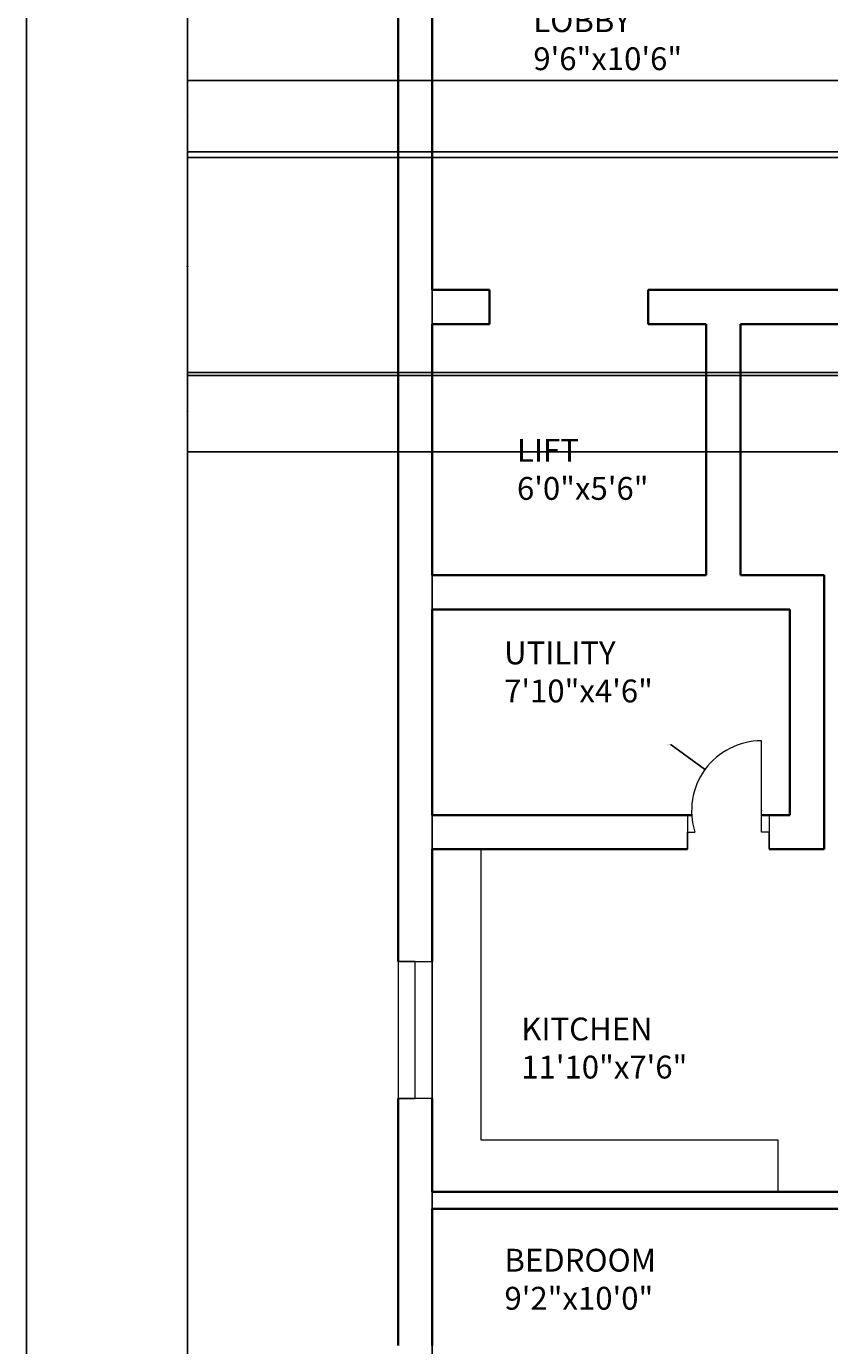
# Model space of a CAD drawing. Units: inches. Extents: x 1902 to 2626, y 1199 to 2408.
# Tile 2 of 9: x 1902 to 2113, y 1470 to 1817. Entities that reach past the tile are written whole.
import ezdxf

# ---------------------------------------------------------------- set-up
doc = ezdxf.new("R2010")
doc.units = ezdxf.units.IN
for name, color, linetype, lineweight in [('A-ANNO-DIMS', 2, 'Continuous', 18), ('A-ANNO-TTLB', 7, 'Continuous', 25), ('A-AREA-IDEN', 7, 'Continuous', 18), ('A-DOOR', 31, 'Continuous', 18), ('A-FLOR-CASE', 8, 'Continuous', 18), ('A-GLAZ', 181, 'Continuous', 18), ('A-WALL', 7, 'Continuous', 35)]:
    doc.layers.add(name, color=color, linetype=linetype, lineweight=lineweight)
doc.styles.get("Standard").update_dxf_attribs({"font": 'arial.ttf'})
doc.dimstyles.get("Standard").update_dxf_attribs({"dimtxt": 0.18, "dimasz": 0.18, "dimexe": 0.18, "dimexo": 0.0625, "dimgap": 0.09, "dimtad": 0, "dimtih": 1, "dimtoh": 1, "dimdec": 4, "dimzin": 0, "dimdsep": 46, "dimtxsty": 'Standard', "dimcen": 0.09, "dimadec": 0, "dimazin": 0, "dimtfac": 1, "dimtdec": 4, "dimtofl": 0, "dimtmove": 0, "dimatfit": 3, "dimfxl": 1, "dimtolj": 1, "dimtzin": 0, "dimarcsym": 0})

# ---------------------------------------------------------------- blocks, each defined once
blk = doc.blocks.new('*D29')
at = {"layer": 'A-ANNO-DIMS', "color": 0, "lineweight": -2, "transparency": 16777216}
for p, q in [((2191.29, 2322.47), (1943.87, 2322.47)), ((1944.05, 2322.29), (1944.05, 1836.38)), ((1944.05, 1350.11), (1944.05, 1836.02)), ((2202.79, 1349.93), (1943.87, 1349.93))]:
    blk.add_line(p, q, dxfattribs=at)
at = {"layer": 'A-ANNO-DIMS', "color": 0, "transparency": 16777216}
for points in [[(1944.02, 2322.29), (1944.08, 2322.29), (1944.05, 2322.47)], [(1944.02, 1350.11), (1944.08, 1350.11), (1944.05, 1349.93)]]:
    blk.add_solid(points, dxfattribs=at)
at = {"layer": 'Defpoints', "color": 0, "transparency": 16777216}
for p in [(1944.05, 2322.47), (2191.35, 2322.47), (2202.85, 1349.93)]:
    blk.add_point(p, dxfattribs=at)
at = {"layer": 'A-ANNO-DIMS', "color": 0, "transparency": 16777216, "insert": (1944.05, 1836.2), "char_height": 0.18, "attachment_point": 5}
blk.add_mtext('\\A1;972.5', dxfattribs=at)
blk = doc.blocks.new('*D38')
at = {"layer": 'A-ANNO-DIMS', "color": 0, "lineweight": -2, "transparency": 16777216}
for p, q in [((2008.35, 1874.05), (2008.35, 1198.67)), ((2128.35, 1874.05), (2128.35, 1198.67)), ((2008.53, 1198.85), (2068.07, 1198.85)), ((2128.17, 1198.85), (2068.63, 1198.85))]:
    blk.add_line(p, q, dxfattribs=at)
at = {"layer": 'A-ANNO-DIMS', "color": 0, "transparency": 16777216}
for points in [[(2008.53, 1198.88), (2008.53, 1198.82), (2008.35, 1198.85)], [(2128.17, 1198.88), (2128.17, 1198.82), (2128.35, 1198.85)]]:
    blk.add_solid(points, dxfattribs=at)
at = {"layer": 'Defpoints', "color": 0, "transparency": 16777216}
for p in [(2008.35, 1874.11), (2128.35, 1874.11), (2128.35, 1198.85)]:
    blk.add_point(p, dxfattribs=at)
at = {"layer": 'A-ANNO-DIMS', "color": 0, "transparency": 16777216, "insert": (2068.35, 1198.85), "char_height": 0.18, "attachment_point": 5}
blk.add_mtext('\\A1;120', dxfattribs=at)
blk = doc.blocks.new('*D40')
at = {"layer": 'A-ANNO-DIMS', "color": 0, "lineweight": -2, "transparency": 16777216}
for p, q in [((2313.55, 1782.51), (1943.87, 1782.51)), ((1944.05, 1782.33), (1944.05, 1754.03)), ((1944.05, 1725.38), (1944.05, 1753.67)), ((2313.55, 1725.2), (1943.87, 1725.2))]:
    blk.add_line(p, q, dxfattribs=at)
at = {"layer": 'A-ANNO-DIMS', "color": 0, "transparency": 16777216}
for points in [[(1944.02, 1782.33), (1944.08, 1782.33), (1944.05, 1782.51)], [(1944.02, 1725.38), (1944.08, 1725.38), (1944.05, 1725.2)]]:
    blk.add_solid(points, dxfattribs=at)
at = {"layer": 'Defpoints', "color": 0, "transparency": 16777216}
for p in [(1944.05, 1782.51), (2313.62, 1782.51), (2313.62, 1725.2)]:
    blk.add_point(p, dxfattribs=at)
at = {"layer": 'A-ANNO-DIMS', "color": 0, "transparency": 16777216, "insert": (1944.05, 1753.85), "char_height": 0.18, "attachment_point": 5}
blk.add_mtext('\\A1;57.31', dxfattribs=at)
blk = doc.blocks.new('*D42')
at = {"layer": 'A-ANNO-DIMS', "color": 0, "lineweight": -2, "transparency": 16777216}
for p, q in [((2267.32, 1726.02), (1943.87, 1726.02)), ((1944.05, 1725.84), (1944.05, 1715.78)), ((1944.05, 1705.36), (1944.05, 1715.41)), ((2267.32, 1705.18), (1943.87, 1705.18))]:
    blk.add_line(p, q, dxfattribs=at)
at = {"layer": 'A-ANNO-DIMS', "color": 0, "transparency": 16777216}
for points in [[(1944.02, 1725.84), (1944.08, 1725.84), (1944.05, 1726.02)], [(1944.02, 1705.36), (1944.08, 1705.36), (1944.05, 1705.18)]]:
    blk.add_solid(points, dxfattribs=at)
at = {"layer": 'Defpoints', "color": 0, "transparency": 16777216}
for p in [(1944.05, 1726.02), (2267.38, 1726.02), (2267.38, 1705.18)]:
    blk.add_point(p, dxfattribs=at)
at = {"layer": 'A-ANNO-DIMS', "color": 0, "transparency": 16777216, "insert": (1944.05, 1715.6), "char_height": 0.18, "attachment_point": 5}
blk.add_mtext('\\A1;20.84', dxfattribs=at)
blk = doc.blocks.new('*D44')
at = {"layer": 'A-ANNO-DIMS', "color": 0, "lineweight": -2, "transparency": 16777216}
for p, q in [((2265.36, 1802.76), (1943.87, 1802.76)), ((1944.05, 1802.58), (1944.05, 1793.54)), ((1944.05, 1784.15), (1944.05, 1793.18)), ((2265.36, 1783.97), (1943.87, 1783.97))]:
    blk.add_line(p, q, dxfattribs=at)
at = {"layer": 'A-ANNO-DIMS', "color": 0, "transparency": 16777216}
for points in [[(1944.02, 1802.58), (1944.08, 1802.58), (1944.05, 1802.76)], [(1944.02, 1784.15), (1944.08, 1784.15), (1944.05, 1783.97)]]:
    blk.add_solid(points, dxfattribs=at)
at = {"layer": 'Defpoints', "color": 0, "transparency": 16777216}
for p in [(1944.05, 1802.76), (2265.42, 1802.76), (2265.42, 1783.97)]:
    blk.add_point(p, dxfattribs=at)
at = {"layer": 'A-ANNO-DIMS', "color": 0, "transparency": 16777216, "insert": (1944.05, 1793.36), "char_height": 0.18, "attachment_point": 5}
blk.add_mtext('\\A1;18.79', dxfattribs=at)
blk = doc.blocks.new('*D58')
at = {"layer": 'A-ANNO-DIMS', "color": 0, "lineweight": -2, "transparency": 16777216}
for p, q in [((2070.93, 1628.13), (2071.11, 1628.13)), ((2071.11, 1628.13), (2079.87, 1621.75)), ((2094.77, 1610.85), (2094.95, 1610.85)), ((2094.86, 1610.76), (2094.86, 1610.94))]:
    blk.add_line(p, q, dxfattribs=at)
at = {"layer": 'A-ANNO-DIMS', "color": 0, "transparency": 16777216}
blk.add_solid([(2079.89, 1621.78), (2079.85, 1621.73), (2080.02, 1621.65)], dxfattribs=at)
at = {"layer": 'Defpoints', "color": 0, "transparency": 16777216}
for p in [(2080.02, 1621.65), (2094.86, 1610.85)]:
    blk.add_point(p, dxfattribs=at)
at = {"layer": 'A-ANNO-DIMS', "color": 0, "transparency": 16777216, "insert": (2070.38, 1628.13), "char_height": 0.18, "attachment_point": 5}
blk.add_mtext('\\A1;R18.356', dxfattribs=at)

msp = doc.modelspace()

# ---------------------------------------------------------------- linework, layer by layer
at = {"layer": 'A-ANNO-TTLB'}
msp.add_lwpolyline([(1901.6928, 2408.1473), (2626.1646, 2408.1473), (2626.1646, 1206.3103), (1901.6928, 1206.3103)], close=True, dxfattribs=at)
at = {"layer": 'A-DOOR'}
for p, q in [((2094.8588, 1605.2028), (2094.8588, 1629.2028)), ((2075.3921, 1609.7028), (2075.3921, 1600.7028)), ((2096.8588, 1609.7028), (2096.8588, 1600.7028)), ((2075.3921, 1600.7028), (2075.3921, 1605.2028)), ((2075.3921, 1605.2028), (2077.3921, 1605.2028)), ((2096.8588, 1605.2028), (2094.8588, 1605.2028)), ((2096.8588, 1600.7028), (2096.8588, 1605.2028))]:
    msp.add_line(p, q, dxfattribs=at)
msp.add_arc((2094.8588, 1610.8468), 18.356, 90, 197.907149, dxfattribs=at)
at = {"layer": 'A-FLOR-CASE'}
for p, q in [((2021.1469, 1600.7028), (2021.1469, 1524.3763)), ((2021.1469, 1524.3763), (2099.2038, 1524.3763)), ((2099.2038, 1524.3763), (2099.2038, 1510.7028))]:
    msp.add_line(p, q, dxfattribs=at)
at = {"layer": 'A-GLAZ'}
for p, q in [((2003.8507, 1571.1752), (1999.3507, 1571.1752)), ((1999.3507, 1571.1752), (2008.3507, 1571.1752)), ((1999.3507, 1571.1752), (1999.3507, 1535.1752)), ((2003.8507, 1535.1752), (2003.8507, 1571.1752)), ((2008.3507, 1571.1752), (2008.3507, 1535.1752)), ((2008.3507, 1535.1752), (1999.3507, 1535.1752)), ((1999.3507, 1535.1752), (2002.8547, 1535.1752)), ((2002.8547, 1535.1752), (2003.8507, 1535.1752))]:
    msp.add_line(p, q, dxfattribs=at)
at = {"layer": 'A-WALL'}
for p, q in [((1999.3507, 2070.6537), (1999.3507, 1571.1752)), ((2008.3507, 2032.9733), (2008.3507, 1747.7028)), ((2023.3497, 1747.7028), (2008.3507, 1747.7028)), ((2023.3497, 1747.7028), (2023.3497, 1738.7028)), ((2089.3507, 1747.7028), (2065.1283, 1747.7028)), ((2065.1283, 1747.7028), (2065.1283, 1747.7028)), ((2065.1283, 1747.7028), (2065.1283, 1738.7028)), ((2091.6431, 1747.7028), (2089.3507, 1747.7028)), ((2128.3507, 1747.7028), (2091.6431, 1747.7028)), ((2008.3507, 1672.7028), (2008.3507, 1738.7028)), ((2008.3507, 1738.7028), (2023.3497, 1738.7028)), ((2008.3507, 1738.7028), (2008.3507, 1672.7028)), ((2065.1283, 1738.7028), (2080.3507, 1738.7028)), ((2080.3507, 1738.7028), (2080.3507, 1672.7028)), ((2089.3507, 1672.7028), (2089.3507, 1738.7028)), ((2137.3507, 1738.7028), (2089.3507, 1738.7028)), ((2008.3507, 1672.7028), (2080.3507, 1672.7028)), ((2089.3507, 1672.7028), (2111.3507, 1672.7028)), ((2111.3507, 1672.7028), (2111.3507, 1663.7028)), ((2008.3507, 1654.7028), (2008.3507, 1663.7028)), ((2008.3507, 1663.7028), (2102.3507, 1663.7028)), ((2008.3507, 1663.7028), (2008.3507, 1609.7028)), ((2102.3507, 1654.7028), (2102.3507, 1663.7028)), ((2111.3507, 1663.7028), (2111.3507, 1600.7028)), ((2102.3507, 1609.7028), (2102.3507, 1654.7028)), ((2076.5385, 1609.7028), (2008.3507, 1609.7028)), ((2102.3507, 1609.7028), (2094.8588, 1609.7028)), ((2111.3507, 1600.7028), (2111.3507, 1609.7028)), ((2008.3507, 1600.7028), (2075.3921, 1600.7028)), ((2008.3507, 1600.7028), (2008.3507, 1571.1752)), ((2008.3507, 1571.1752), (2008.3507, 1600.7028)), ((2096.8588, 1600.7028), (2102.3507, 1600.7028)), ((2111.3507, 1600.7028), (2102.3507, 1600.7028)), ((2102.3507, 1600.7028), (2102.3507, 1600.7028)), ((2102.3507, 1600.7028), (2111.3507, 1600.7028)), ((1999.3507, 1535.1752), (1999.3507, 1470.2482)), ((2008.3507, 1510.7028), (2008.3507, 1535.1752)), ((2008.3507, 1535.1752), (2008.3507, 1510.7028)), ((2207.3507, 1510.7028), (2008.3507, 1510.7028)), ((2008.3507, 1506.2028), (2118.3507, 1506.2028)), ((2008.3507, 1506.2028), (2008.3507, 1470.2482))]:
    msp.add_line(p, q, dxfattribs=at)

# ---------------------------------------------------------------- texts
at = {"layer": 'A-AREA-IDEN', "char_height": 6, "attachment_point": 1}
for s, width, insert in [('LOBBY\\P9\'6"x10\'6"', 191.395477, (2034.9094, 1821.4733)), ('LIFT\\P6\'0"x5\'6"', 140.584417, (2030.6102, 1708.5441)), ('UTILITY\\P7\'10"x4\'6"', 121.557168, (2027.2249, 1655.307)), ('KITCHEN\\P11\'10"x7\'6"', 170.105713, (2031.7385, 1556.4526)), ('BEDROOM\\P9\'2"x10\'0"', 128.780928, (2027.3209, 1495.6957))]:
    msp.add_mtext_dynamic_manual_height_columns(s, width=width, gutter_width=12.5, heights=[0], dxfattribs=dict(at, insert=insert))

# ---------------------------------------------------------------- dimensions: what is measured, and where the dimension line sits
at = {"layer": 'A-ANNO-DIMS'}
for base, p1, p2, override, picture, middle in [((1944.0507, 2322.4733), (2202.8507, 1349.9322), (2191.3507, 2322.4733), {"dimdec": 1, "dimlfac": 1, "dimrnd": 0, "dimzin": 0, "dimdsep": 46, "dimlunit": 2}, '*D29', (1944.0507, 1836.2028)), ((1944.0507, 1802.7563), (2265.4197, 1783.9667), (2265.4197, 1802.7563), {"dimdec": 2, "dimlfac": 1, "dimrnd": 0, "dimzin": 0, "dimdsep": 46, "dimlunit": 2}, '*D44', (1944.0507, 1793.3615)), ((1944.0507, 1782.5063), (2313.6163, 1725.1982), (2313.6163, 1782.5063), {"dimdec": 2, "dimlfac": 1, "dimrnd": 0, "dimzin": 0, "dimdsep": 46, "dimlunit": 2}, '*D40', (1944.0507, 1753.8523)), ((1944.0507, 1726.0164), (2267.379, 1705.1771), (2267.379, 1726.0164), {"dimdec": 2, "dimlfac": 1, "dimrnd": 0, "dimzin": 0, "dimdsep": 46, "dimlunit": 2}, '*D42', (1944.0507, 1715.5967))]:
    dim = msp.add_linear_dim(base=base, p1=p1, p2=p2, angle=90, dimstyle='Standard', override=override, dxfattribs=at)
    dim.commit()
    dim.dimension.update_dxf_attribs({"geometry": picture, "text_midpoint": middle})
dim = msp.add_linear_dim(base=(2128.3507, 1198.8475), p1=(2008.3507, 1874.11), p2=(2128.3507, 1874.11), dimstyle='Standard', override={"dimdec": 0, "dimlfac": 1, "dimrnd": 0, "dimzin": 0, "dimdsep": 46, "dimlunit": 2}, dxfattribs=at)
dim.commit()
dim.dimension.update_dxf_attribs({"geometry": '*D38', "text_midpoint": (2068.3507, 1198.8475)})
dim = msp.add_radius_dim(center=(2094.8588, 1610.8468), mpoint=(2080.0171, 1621.6479), dimstyle='Standard', override={"dimdec": 3, "dimlfac": 1, "dimrnd": 0, "dimzin": 0, "dimdsep": 46, "dimlunit": 2}, dxfattribs=at)
dim.commit()
dim.dimension.update_dxf_attribs({"geometry": '*D58', "text_midpoint": (2070.3823, 1628.1286), "dimtype": 164})

doc.saveas('drawing.dxf')
